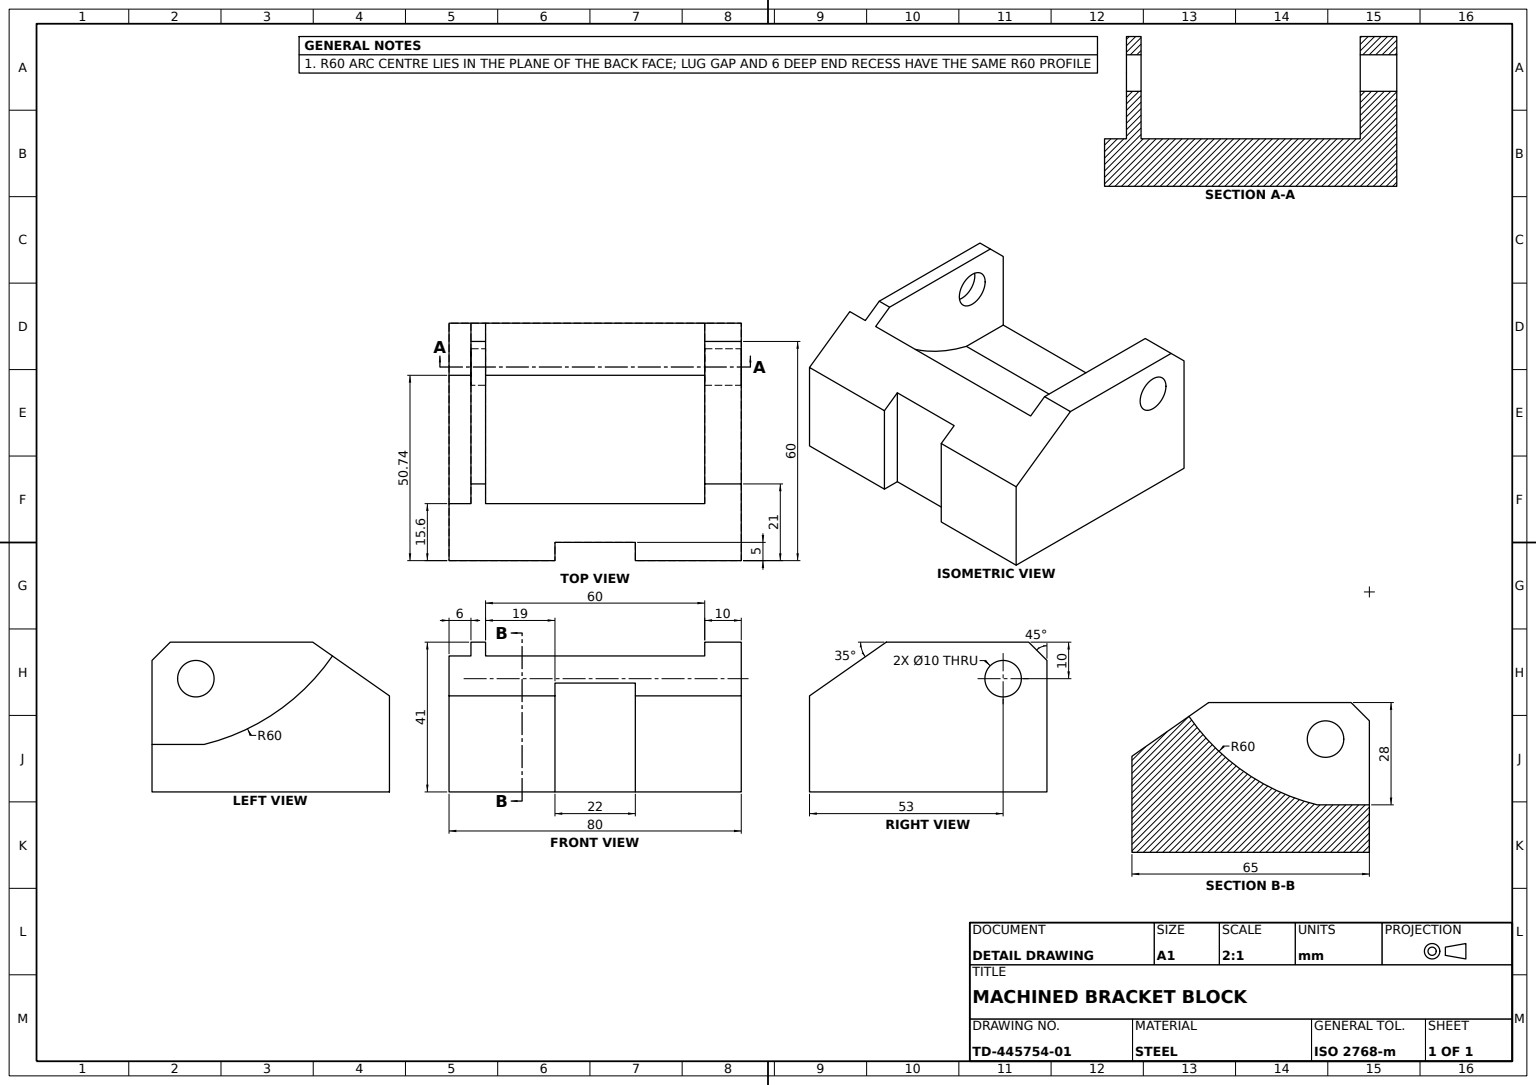
SolidWorks part; units mm, degrees
material "Plain Carbon Steel"
ref_plane "Front Plane" through (0, 0, 0) normal (0, 0, 1) x (1, 0, 0)
ref_plane "Top Plane" through (0, 0, 0) normal (0, 1, 0) x (1, 0, 0)
ref_plane "Right Plane" through (0, 0, 0) normal (1, 0, 0) x (0, 0, -1)
sketch "Block Profile Sketch" plane through (0, 0, 0) normal (0, 0, 1) x (1, 0, 0)
  line L1 (0, 0) -> (65, 0)
  line L2 (0, 0) -> (0, 41)
  line L3 (0, 41) -> (65, 41)
  line L4 (65, 0) -> (65, 41)
  circle A0 centre (12, 31) radius 5
  dimension "D5" = 10
  dimension "D1" = 65
  dimension "D2" = 41
  dimension "D3" = 10
  dimension "D4" = 12
extrude "Block Body 80mm" add sketch "Block Profile Sketch" along normal mid plane 80
chamfer "Edge Chamfer 5mm" distance 5 angle 45 1 edges at (0, 41, 0)
chamfer "Top Chamfer 21mm x 35deg" distance 21 angle 35 1 edges at (65, 41, 0)
sketch "Top Recess Sketch" plane through (0, 0, 40) normal (0, 0, 1) x (1, 0, 0)
  line L1 (0, 36) -> (0, 0) construction
  line L2 (0, 13) -> (14.2646, 13)
  line L3 (65, 0) -> (65, 26.2956) construction
  line L4 (44, 41) -> (5, 41) construction
  line L10 (0, 13) -> (0, 36)
  line L11 (0, 36) -> (5, 41)
  line L12 (5, 41) -> (44, 41)
  line L13 (44, 41) -> (49.3966, 37.2213)
  arc A0 (14.2646, 13) -> (49.3966, 37.2213) centre (0, 71.2797) ccw
  dimension "D3" = 120
  dimension "D1" = 28
  dimension "D2" = 14.2646
  dimension "D4" = 15.6034
extrude "Top Recess Cut 6mm" cut sketch "Top Recess Sketch" against normal blind 6
ref_plane "Lug Gap Plane Offset 10mm" through (0, 0, 30) normal (0, 0, 1) x (1, 0, 0)
sketch "Lug Gap Sketch" plane through (0, 0, 30) normal (0, 0, 1) x (1, 0, 0)
  line L0 (0, 13) -> (0, 36)
  line L1 (0, 36) -> (5, 41)
  line L2 (5, 41) -> (44, 41)
  line L3 (44, 41) -> (49.3966, 37.2213)
  line L4 (0, 13) -> (14.2646, 13)
  line L5 (48.7929, 37.644) -> (49.3966, 37.2213)
  arc A1 (14.2646, 13) -> (49.3966, 37.2213) centre (0, 71.2797) ccw
  dimension "D1" = 120
  dimension "D2" = 5
  dimension "D3" = 14.2646
  dimension "D4" = 23
  dimension "D5" = 48.7929
  dimension "D6" = 49.3966
  dimension "D7" = 24.644
extrude "Lug Gap Cut 60mm" cut sketch "Lug Gap Sketch" against normal blind 60 contours A1 L4 L0 L1 L2 L3
sketch "Through Slot Sketch" plane through (0, 41, 0) normal (0, 1, 0) x (1, 0, 0)
  line L0 (65, 40) -> (65, -40) construction
  line L1 (65, 11) -> (60, 11)
  line L2 (65, 11) -> (65, -11)
  line L3 (65, -11) -> (60, -11)
  line L4 (60, 11) -> (60, -11)
  line L5 (0, 0) -> (93.9874, 0)
  line L6 (0, 30) -> (0, -30) construction
  line L7 (44, 30) -> (44, 40) construction
  dimension "D1" = 22
  dimension "D2" = 11
  dimension "D3" = 5
  dimension "D4" = 49.9874
extrude "Through Slot Cut" cut sketch "Through Slot Sketch" against normal blind 210 contours L2 L3 L4 L1
